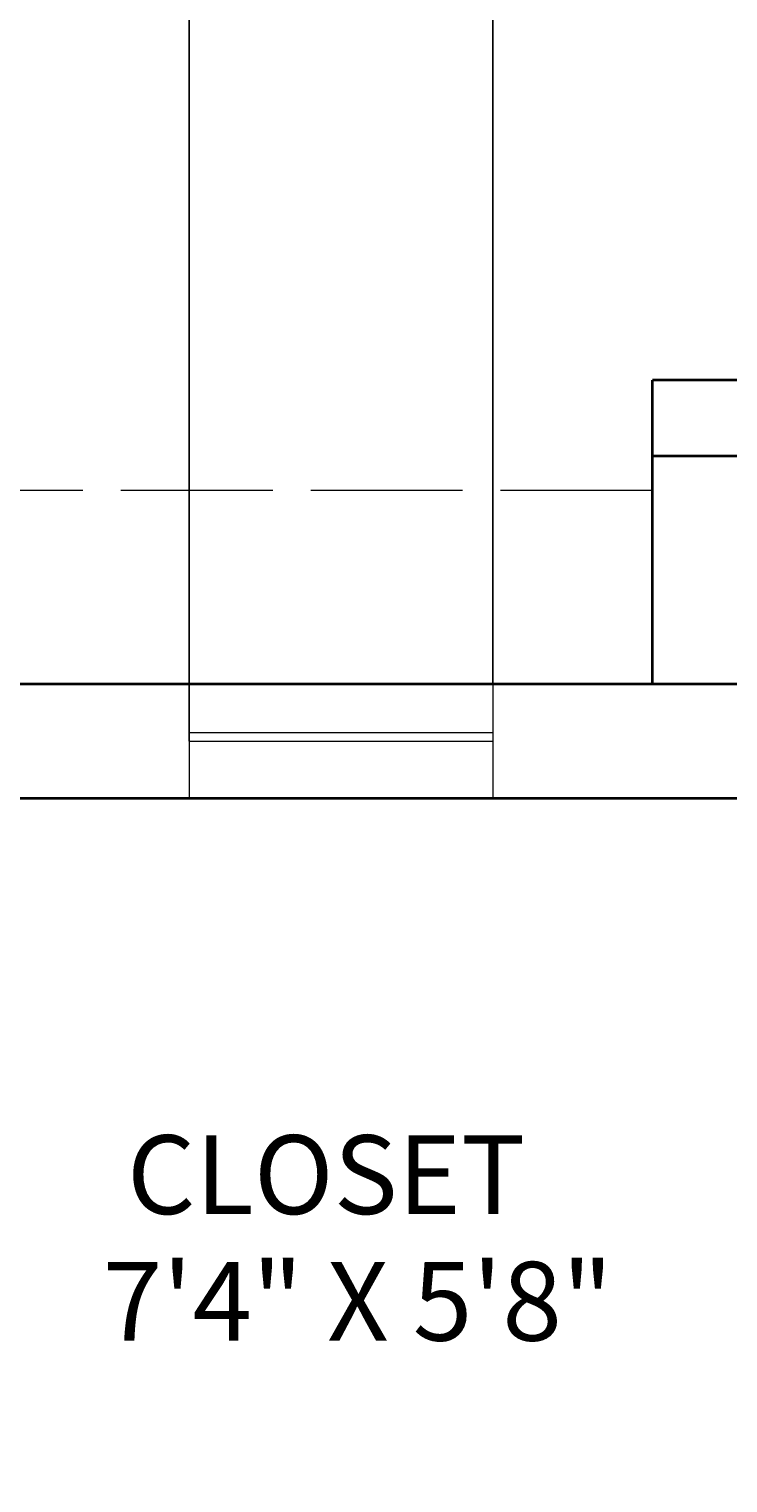
# Model space of a CAD drawing. Units: inches. Extents: x -61 to 1599, y -1316 to 257.
# Tile 68 of 204: x 240 to 295, y -680 to -565. Entities that reach past the tile are written whole.
import ezdxf

# ---------------------------------------------------------------- set-up
doc = ezdxf.new("R2010")
doc.units = ezdxf.units.IN
doc.header["$MEASUREMENT"] = 0
doc.linetypes.add('ACAD_ISO02W100', pattern=[15, 12, -3])
for name, color, linetype, lineweight in [('A-ANNO-DIMS', 2, 'Continuous', 18), ('A-AREA-IDEN', 1, 'Continuous', 18), ('A-FLOR-OVHD', 203, 'ACAD_ISO02W100', 13), ('WALLS', 4, 'Continuous', 35), ('WINDOWS', 220, 'Continuous', 18)]:
    doc.layers.add(name, color=color, linetype=linetype, lineweight=lineweight)
doc.styles.get("Standard").update_dxf_attribs({"font": 'arial.ttf'})
doc.dimstyles.get("Standard").update_dxf_attribs({"dimtxt": 0.18, "dimasz": 0.18, "dimexe": 0.18, "dimexo": 0.0625, "dimgap": 0.09, "dimtad": 0, "dimtih": 1, "dimtoh": 1, "dimdec": 0, "dimzin": 0, "dimdsep": 46, "dimlunit": 3, "dimtxsty": 'Standard', "dimcen": 0.09, "dimadec": 0, "dimazin": 0, "dimtfac": 1, "dimtdec": 0, "dimtofl": 0, "dimtmove": 0, "dimatfit": 3, "dimfxl": 1, "dimtolj": 1, "dimtzin": 0, "dimarcsym": 0})

# ---------------------------------------------------------------- blocks, each defined once
blk = doc.blocks.new('WIN-24IN')
for p, q in [((0, 4.5), (0, 9)), ((0, 9), (0, 0)), ((24, 9), (24, 0)), ((0, 5.19), (24, 5.19)), ((0, 4.5), (24, 4.5))]:
    blk.add_line(p, q)
blk = doc.blocks.new('*D687')
at = {"layer": 'A-ANNO-DIMS', "color": 0, "lineweight": -2, "transparency": 16777216}
for p, q in [((289.42, 181.68), (-61.08, 181.68)), ((-60.9, 181.5), (-60.9, -528.95)), ((-60.9, -1239.76), (-60.9, -529.32)), ((319.64, -1239.94), (-61.08, -1239.94))]:
    blk.add_line(p, q, dxfattribs=at)
at = {"layer": 'A-ANNO-DIMS', "color": 0, "transparency": 16777216}
for points in [[(-60.93, 181.5), (-60.87, 181.5), (-60.9, 181.68)], [(-60.93, -1239.76), (-60.87, -1239.76), (-60.9, -1239.94)]]:
    blk.add_solid(points, dxfattribs=at)
at = {"layer": 'DEFPOINTS', "color": 0, "transparency": 16777216}
for p in [(289.48, 181.68), (-60.9, -1239.94), (319.7, -1239.94)]:
    blk.add_point(p, dxfattribs=at)
at = {"layer": 'A-ANNO-DIMS', "color": 0, "transparency": 16777216, "insert": (-60.9, -529.13), "char_height": 0.18, "attachment_point": 5}
blk.add_mtext('\\A1;1421.6', dxfattribs=at)
blk = doc.blocks.new('*D701')
at = {"layer": 'A-ANNO-DIMS', "color": 0, "lineweight": -2, "transparency": 16777216}
for p, q in [((215.75, -616.88), (215.75, 257.46)), ((215.93, 257.28), (233.92, 257.28)), ((252.7, 257.28), (234.71, 257.28)), ((252.88, -616.88), (252.88, 257.46))]:
    blk.add_line(p, q, dxfattribs=at)
at = {"layer": 'A-ANNO-DIMS', "color": 0, "transparency": 16777216}
for points in [[(215.93, 257.31), (215.93, 257.25), (215.75, 257.28)], [(252.7, 257.31), (252.7, 257.25), (252.88, 257.28)]]:
    blk.add_solid(points, dxfattribs=at)
at = {"layer": 'DEFPOINTS', "color": 0, "transparency": 16777216}
for p in [(252.88, 257.28), (215.75, -616.94), (252.88, -616.94)]:
    blk.add_point(p, dxfattribs=at)
at = {"layer": 'A-ANNO-DIMS', "color": 0, "transparency": 16777216, "insert": (234.32, 257.28), "char_height": 0.18, "attachment_point": 5}
blk.add_mtext('\\A1;37.13', dxfattribs=at)
blk = doc.blocks.new('*D702')
at = {"layer": 'A-ANNO-DIMS', "color": 0, "lineweight": -2, "transparency": 16777216}
for p, q in [((276.88, -616.88), (276.88, 257.46)), ((277.06, 257.28), (312.21, 257.28)), ((348.14, 257.28), (312.99, 257.28)), ((348.32, -616.88), (348.32, 257.46))]:
    blk.add_line(p, q, dxfattribs=at)
at = {"layer": 'A-ANNO-DIMS', "color": 0, "transparency": 16777216}
for points in [[(277.06, 257.31), (277.06, 257.25), (276.88, 257.28)], [(348.14, 257.31), (348.14, 257.25), (348.32, 257.28)]]:
    blk.add_solid(points, dxfattribs=at)
at = {"layer": 'DEFPOINTS', "color": 0, "transparency": 16777216}
for p in [(348.32, 257.28), (276.88, -616.94), (348.32, -616.94)]:
    blk.add_point(p, dxfattribs=at)
at = {"layer": 'A-ANNO-DIMS', "color": 0, "transparency": 16777216, "insert": (312.6, 257.28), "char_height": 0.18, "attachment_point": 5}
blk.add_mtext('\\A1;71.44', dxfattribs=at)

msp = doc.modelspace()

# ---------------------------------------------------------------- linework, layer by layer
at = {"layer": 'A-FLOR-OVHD'}
msp.add_line((289.4807, -601.6522), (160.8585, -601.6522), dxfattribs=at)
at = {"layer": 'WALLS'}
for p, q in [((289.4807, -616.9446), (289.4807, -592.9446)), ((403.7028, -592.9446), (289.4807, -592.9446)), ((403.7028, -598.9446), (289.4807, -598.9446)), ((544.7028, -616.9446), (14.7028, -616.9446)), ((237.7028, -625.9446), (321.7028, -625.9446))]:
    msp.add_line(p, q, dxfattribs=at)

# ---------------------------------------------------------------- block references
at = {"layer": 'WINDOWS'}
msp.add_blockref('WIN-24IN', (252.882, -625.9447), dxfattribs=at)

# ---------------------------------------------------------------- texts
at = {"layer": 'A-AREA-IDEN'}
for s, height, p in [('   CLOSET', 6.22364, (242.2634, -658.7715)), ('  7\'4" X 5\'8"', 6.223643, (242.2634, -668.7692))]:
    msp.add_text(s, height=height, dxfattribs=at).set_placement(p)

# ---------------------------------------------------------------- dimensions: what is measured, and where the dimension line sits
at = {"layer": 'A-ANNO-DIMS'}
for base, p1, p2, picture, middle in [((252.8825, 257.2771), (215.7521, -616.9446), (252.8825, -616.9446), '*D701', (234.3173, 257.2771)), ((348.3201, 257.2771), (276.8825, -616.9446), (348.3201, -616.9446), '*D702', (312.6013, 257.2771))]:
    dim = msp.add_linear_dim(base=base, p1=p1, p2=p2, dimstyle='Standard', override={"dimdec": 2, "dimlfac": 1, "dimrnd": 0, "dimzin": 0, "dimdsep": 46, "dimlunit": 2}, dxfattribs=at)
    dim.commit()
    dim.dimension.update_dxf_attribs({"geometry": picture, "text_midpoint": middle})
dim = msp.add_linear_dim(base=(-60.8972, -1239.9446), p1=(289.4807, 181.6771), p2=(319.7028, -1239.9446), angle=90, dimstyle='Standard', override={"dimdec": 1, "dimlfac": 1, "dimrnd": 0, "dimzin": 0, "dimdsep": 46, "dimlunit": 2}, dxfattribs=at)
dim.commit()
dim.dimension.update_dxf_attribs({"geometry": '*D687', "text_midpoint": (-60.8972, -529.1337)})

doc.saveas('drawing.dxf')
